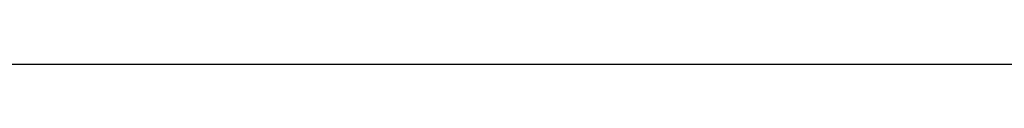
# Model space of a CAD drawing. Units: inches. Extents: x 459864 to 460310, y 324185 to 324787.
# Tile 101 of 112: x 460248.739 to 460250.864, y 324283.483 to 324283.483. Entities that reach past the tile are written whole.
import ezdxf

# ---------------------------------------------------------------- set-up
doc = ezdxf.new("R2010")
doc.units = ezdxf.units.IN
doc.layers.add('A-ANNO-DIMS', color=2, linetype='Continuous', lineweight=18)
doc.styles.get("Standard").update_dxf_attribs({"font": 'arial.ttf'})
doc.dimstyles.new('ISO-25', dxfattribs={"dimtxt": 6, "dimasz": 2.5, "dimexe": 1.25, "dimexo": 0.625, "dimtad": 1, "dimdec": 1, "dimlunit": 3, "dimtxsty": 'Standard', "dimcen": 2.5, "dimadec": 0, "dimazin": 0, "dimtfac": 1, "dimtdec": 1, "dimtmove": 0, "dimatfit": 3, "dimfxl": 1, "dimarcsym": 0})

# ---------------------------------------------------------------- blocks, each defined once
blk = doc.blocks.new('*D21')
at = {"layer": 'A-ANNO-DIMS', "color": 0, "lineweight": -2, "transparency": 16777216}
for p, q in [((460247.7399, 324715.4832), (460309.5804, 324715.4832)), ((460308.3304, 324712.9832), (460308.3304, 324285.9832)), ((460247.7399, 324283.4832), (460309.5804, 324283.4832))]:
    blk.add_line(p, q, dxfattribs=at)
at = {"layer": 'A-ANNO-DIMS', "color": 0, "transparency": 16777216}
for points in [[(460307.9137, 324712.9832), (460308.747, 324712.9832), (460308.3304, 324715.4832)], [(460307.9137, 324285.9832), (460308.747, 324285.9832), (460308.3304, 324283.4832)]]:
    blk.add_solid(points, dxfattribs=at)
at = {"layer": 'Defpoints', "color": 0, "transparency": 16777216}
for p in [(460247.1149, 324715.4832), (460247.1149, 324283.4832), (460308.3304, 324283.4832)]:
    blk.add_point(p, dxfattribs=at)
at = {"layer": 'A-ANNO-DIMS', "color": 0, "transparency": 16777216, "insert": (460304.6399, 324499.4832), "char_height": 6, "attachment_point": 5, "rotation": 90}
blk.add_mtext("36'", dxfattribs=at)
blk = doc.blocks.new('*D62')
at = {"layer": 'A-ANNO-DIMS', "color": 0, "lineweight": -2, "transparency": 16777216}
for p, q in [((460247.7399, 324332.7387), (460278.7649, 324332.7387)), ((460277.5149, 324330.2387), (460277.5149, 324285.9832)), ((460247.7399, 324283.4832), (460278.7649, 324283.4832))]:
    blk.add_line(p, q, dxfattribs=at)
at = {"layer": 'A-ANNO-DIMS', "color": 0, "transparency": 16777216}
for points in [[(460277.0983, 324330.2387), (460277.9316, 324330.2387), (460277.5149, 324332.7387)], [(460277.0983, 324285.9832), (460277.9316, 324285.9832), (460277.5149, 324283.4832)]]:
    blk.add_solid(points, dxfattribs=at)
at = {"layer": 'Defpoints', "color": 0, "transparency": 16777216}
for p in [(460247.1149, 324332.7387), (460247.1149, 324283.4832), (460277.5149, 324283.4832)]:
    blk.add_point(p, dxfattribs=at)
at = {"layer": 'A-ANNO-DIMS', "color": 0, "transparency": 16777216, "insert": (460273.7876, 324308.111), "char_height": 6, "attachment_point": 5, "rotation": 90}
blk.add_mtext('4\'-1 1/2"', dxfattribs=at)
blk = doc.blocks.new('*D65')
at = {"layer": 'A-ANNO-DIMS', "color": 0, "lineweight": -2, "transparency": 16777216}
for p, q in [((460247.7399, 324283.4832), (460302.7649, 324283.4832)), ((460301.5149, 324280.9832), (460301.5149, 324197.4832)), ((460271.7399, 324194.9832), (460302.7649, 324194.9832))]:
    blk.add_line(p, q, dxfattribs=at)
at = {"layer": 'A-ANNO-DIMS', "color": 0, "transparency": 16777216}
for points in [[(460301.0983, 324280.9832), (460301.9316, 324280.9832), (460301.5149, 324283.4832)], [(460301.0983, 324197.4832), (460301.9316, 324197.4832), (460301.5149, 324194.9832)]]:
    blk.add_solid(points, dxfattribs=at)
at = {"layer": 'Defpoints', "color": 0, "transparency": 16777216}
for p in [(460247.1149, 324283.4832), (460271.1149, 324194.9832), (460301.5149, 324194.9832)]:
    blk.add_point(p, dxfattribs=at)
at = {"layer": 'A-ANNO-DIMS', "color": 0, "transparency": 16777216, "insert": (460297.7876, 324239.2332), "char_height": 6, "attachment_point": 5, "rotation": 90}
blk.add_mtext('7\'-4 1/2"', dxfattribs=at)

msp = doc.modelspace()

# ---------------------------------------------------------------- dimensions: what is measured, and where the dimension line sits
at = {"layer": 'A-ANNO-DIMS'}
for base, p1, p2, angle, override, picture, middle in [((460308.3304, 324283.4832), (460247.1149, 324715.4832), (460247.1149, 324283.4832), 90, {"dimclrd": 0, "dimclre": 0, "dimclrt": 0}, '*D21', (460304.6399, 324499.4832)), ((460277.5149, 324283.4832), (460247.1149, 324332.7387), (460247.1149, 324283.4832), 270, {"dimdec": 1, "dimlfac": 1, "dimrnd": 0, "dimzin": 1, "dimdsep": 46, "dimlunit": 4, "dimfrac": 2}, '*D62', (460273.7876, 324308.111)), ((460301.5149, 324194.9832), (460247.1149, 324283.4832), (460271.1149, 324194.9832), 90, {"dimdec": 1, "dimlfac": 1, "dimrnd": 0, "dimzin": 1, "dimdsep": 46, "dimlunit": 4, "dimfrac": 2}, '*D65', (460297.7876, 324239.2332))]:
    dim = msp.add_linear_dim(base=base, p1=p1, p2=p2, angle=angle, dimstyle='ISO-25', override=override, dxfattribs=at)
    dim.commit()
    dim.dimension.update_dxf_attribs({"geometry": picture, "text_midpoint": middle})

doc.saveas('drawing.dxf')
